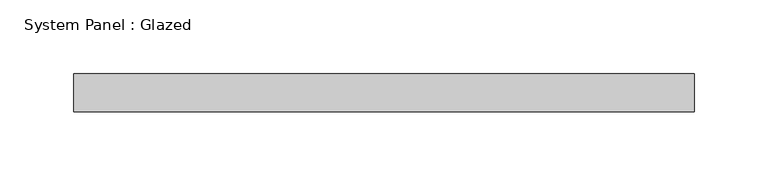
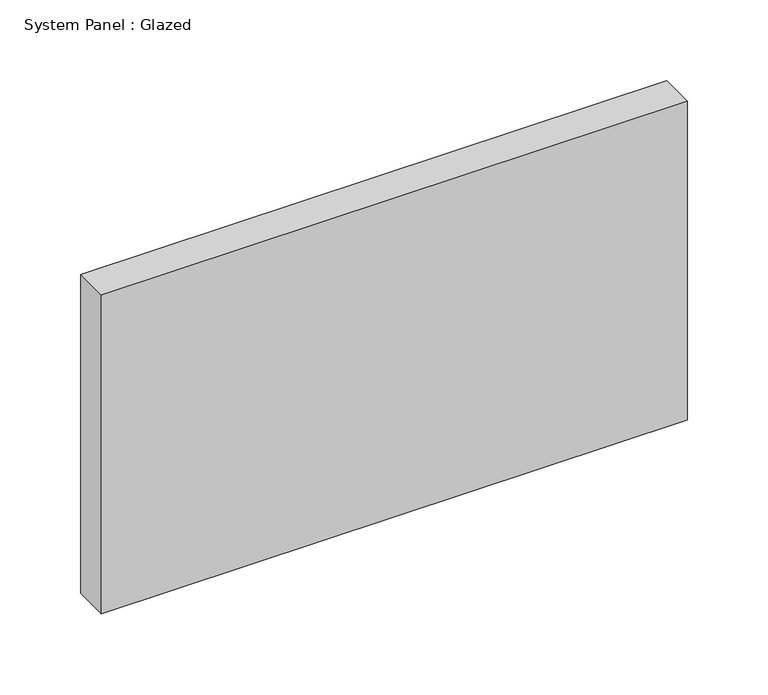
"""IFC4 building model written with IfcOpenShell, lengths in millimetres: plate geometry, System Panel : Glazed."""

from ifc_helpers import new_model, si_unit, origin, origin_with_axes, place, context, project, spatial, polyline, outline, extrude, source, transform, mapped, element, save


def system_panel_glazed_0f3faf12(model_context):
    return source(origin(), model_context, "Body", "SweptSolid", [
        extrude(outline(polyline([(209.55, 19.05), (-209.55, 19.05), (-209.55, 44.45), (209.55, 44.45), (209.55, 19.05)])), origin_with_axes(), (0.0, 0.0, 1.0), 241.3),
    ])


if __name__ == "__main__":
    model = new_model("IFC4")
    model_context = context("Model", 3, world=origin())
    ifc_project = project(units=[si_unit("LENGTHUNIT", "METRE", prefix="MILLI")], contexts=[model_context])
    site = spatial("IfcSite", under=ifc_project)
    building = spatial("IfcBuilding", under=site)
    placement = place(None, origin())
    system_panel_glazed_shape = system_panel_glazed_0f3faf12(model_context)
    element("IfcPlate", 1, ObjectType="System Panel : Glazed", at=placement, inside=building, context=model_context, shape_type="MappedRepresentation", body=[
        mapped(system_panel_glazed_shape, transform((0.0, 0.0, 0.0), x_axis=(1.0, 0.0, 0.0), y_axis=(0.0, 1.0, 0.0), z_axis=(0.0, 0.0, 1.0))),
    ])
    save(model, "model.ifc")

# Revit data of these elements
# Type "System Panel : Glazed"
#   Construction Type Id = "GSP4R"
#   Analytic Construction = "1/8 in Pilkington single glazing"
#   Visual Light Transmittance = 0.9
#   Solar Heat Gain Coefficient = 0.86
#   Heat Transfer Coefficient (U) = 1.18115 BTU/(h·ft²·°F)
#   Define Thermal Properties by = 1
# Element 1 (IfcPlate, "System Panel : Glazed")
#   Materials on its faces: "Glass"
# Materials
#   "Glass": class "Glass", colour RGB 0 128 192, transparency 0.75, Description = "Soda Lime Glass", Cost = 0
